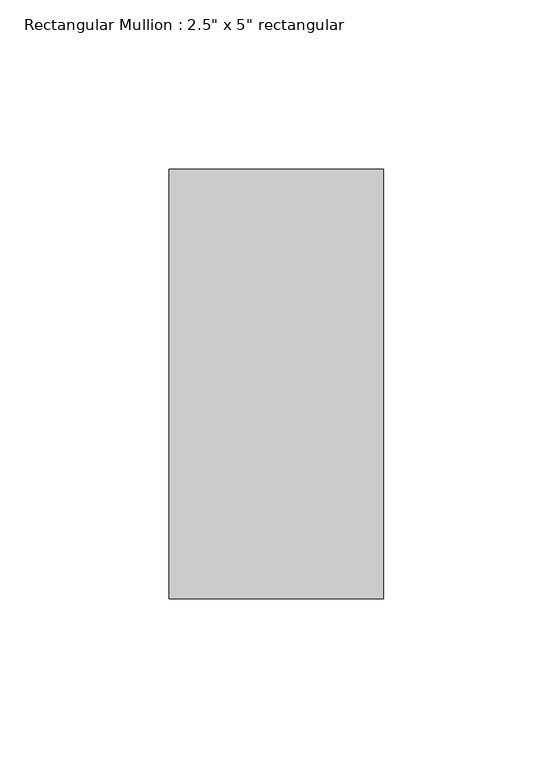
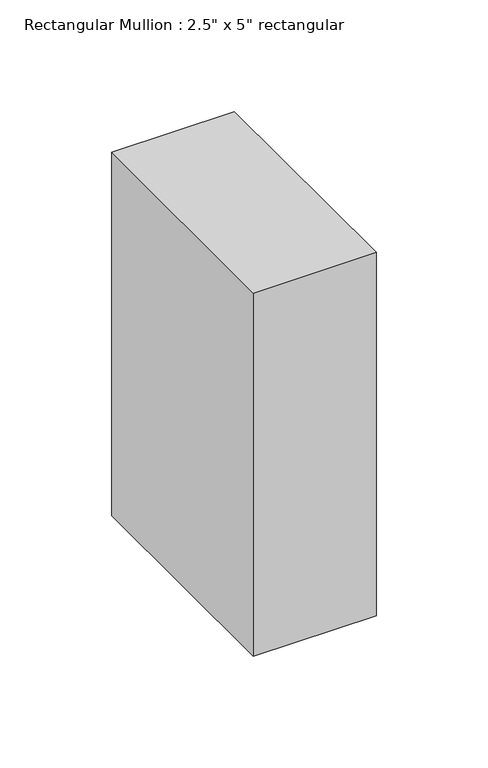
"""IFC4 building model written with IfcOpenShell, lengths in millimetres: member geometry."""

from ifc_helpers import new_model, si_unit, frame, origin, place, context, project, spatial, polyline, outline, extrude, source, transform, mapped, element, save


def member_3782c11a(model_context):
    return source(origin(), model_context, "Body", "SweptSolid", [
        extrude(outline(polyline([(0.0, 63.5), (0.0, -63.5), (-63.5, -63.5), (-63.5, 63.5), (0.0, 63.5)])), frame((0.0, 0.0, -198.755), z_axis=(0.0, 0.0, 1.0), x_axis=(1.0, 0.0, 0.0)), (0.0, 0.0, 1.0), 198.755),
    ])


if __name__ == "__main__":
    model = new_model("IFC4")
    model_context = context("Model", 3, world=origin())
    ifc_project = project(units=[si_unit("LENGTHUNIT", "METRE", prefix="MILLI")], contexts=[model_context])
    site = spatial("IfcSite", under=ifc_project)
    building = spatial("IfcBuilding", under=site)
    placement = place(None, origin())
    member_shape = member_3782c11a(model_context)
    element("IfcMember", 1, ObjectType="Rectangular Mullion : 2.5\" x 5\" rectangular", at=placement, inside=building, context=model_context, shape_type="MappedRepresentation", body=[
        mapped(member_shape, transform((0.0, 0.0, 0.0), x_axis=(1.0, 0.0, 0.0), y_axis=(0.0, 1.0, 0.0), z_axis=(0.0, 0.0, 1.0))),
    ])
    save(model, "model.ifc")

# Revit data of these elements
# Type "Rectangular Mullion : 2.5\" x 5\" rectangular"
#   built-in parameter 1007304 = 0.416667 (stored number, unit not read)
#   built-in parameter 1007301 = 0.104167 (stored number, unit not read)
#   built-in parameter 1007300 = 0.104167 (stored number, unit not read)
# Element 1 (IfcMember, "Rectangular Mullion : 2.5\" x 5\" rectangular")
#   Materials on its faces: "Aluminum"
# Materials
#   "Aluminum": class "Metal", colour RGB 247 247 247, transparency 0, Description = "Aluminum 6061", Cost = 0
